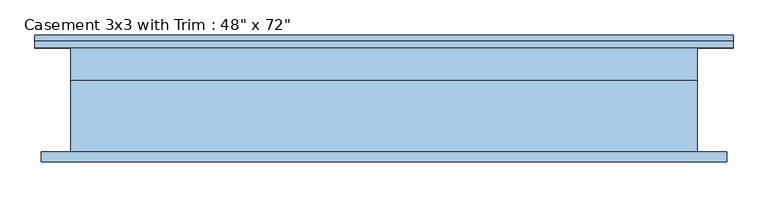
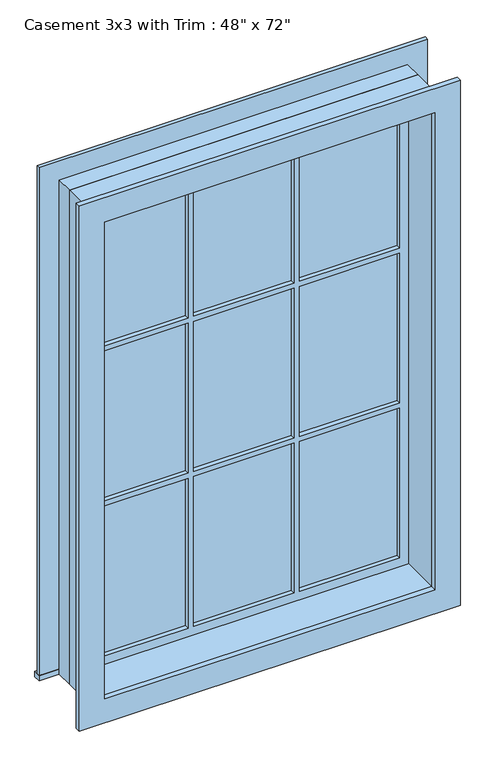
"""IFC4 building model written with IfcOpenShell, lengths in millimetres: window geometry."""

from ifc_helpers import new_model, si_unit, frame, origin, place, context, project, spatial, polyline, outline, extrude, source, transform, mapped, element, save


def window_5a4e61ec(model_context):
    return source(origin(), model_context, "Body", "SweptSolid", [
        extrude(outline(polyline([(-679.45, 127.0), (679.45, 127.0), (679.45, 101.6), (-679.45, 101.6), (-679.45, 127.0)])), frame((0.0, 0.0, 304.8), z_axis=(0.0, 0.0, 1.0), x_axis=(1.0, 0.0, 0.0)), (0.0, 0.0, 1.0), 19.05),
        extrude(outline(polyline([(2114.55, -590.55), (2114.55, 590.55), (323.85, 590.55), (323.85, 679.45), (2203.45, 679.45), (2203.45, -679.45), (323.85, -679.45), (323.85, -590.55), (2114.55, -590.55)])), frame((0.0, 101.6, 0.0), z_axis=(0.0, 1.0, 0.0), x_axis=(0.0, 0.0, 1.0)), (0.0, 0.0, 1.0), 12.7),
        extrude(outline(polyline([(194.7333333, 66.675), (546.1, 66.675), (546.1, 53.975), (194.7333333, 53.975), (194.7333333, 66.675)])), frame((0.0, 0.0, 1515.5333333), z_axis=(0.0, 0.0, 1.0), x_axis=(1.0, 0.0, 0.0)), (0.0, 0.0, 1.0), 554.5666667),
        extrude(outline(polyline([(-175.6833333, 66.675), (175.6833333, 66.675), (175.6833333, 53.975), (-175.6833333, 53.975), (-175.6833333, 66.675)])), frame((0.0, 0.0, 1515.5333333), z_axis=(0.0, 0.0, 1.0), x_axis=(1.0, 0.0, 0.0)), (0.0, 0.0, 1.0), 554.5666667),
        extrude(outline(polyline([(-546.1, 66.675), (-194.7333333, 66.675), (-194.7333333, 53.975), (-546.1, 53.975), (-546.1, 66.675)])), frame((0.0, 0.0, 1515.5333333), z_axis=(0.0, 0.0, 1.0), x_axis=(1.0, 0.0, 0.0)), (0.0, 0.0, 1.0), 554.5666667),
        extrude(outline(polyline([(-546.1, 66.675), (-194.7333333, 66.675), (-194.7333333, 53.975), (-546.1, 53.975), (-546.1, 66.675)])), frame((0.0, 0.0, 941.9166667), z_axis=(0.0, 0.0, 1.0), x_axis=(1.0, 0.0, 0.0)), (0.0, 0.0, 1.0), 554.5666667),
        extrude(outline(polyline([(-175.6833333, 66.675), (175.6833333, 66.675), (175.6833333, 53.975), (-175.6833333, 53.975), (-175.6833333, 66.675)])), frame((0.0, 0.0, 941.9166667), z_axis=(0.0, 0.0, 1.0), x_axis=(1.0, 0.0, 0.0)), (0.0, 0.0, 1.0), 554.5666667),
        extrude(outline(polyline([(194.7333333, 66.675), (546.1, 66.675), (546.1, 53.975), (194.7333333, 53.975), (194.7333333, 66.675)])), frame((0.0, 0.0, 941.9166667), z_axis=(0.0, 0.0, 1.0), x_axis=(1.0, 0.0, 0.0)), (0.0, 0.0, 1.0), 554.5666667),
        extrude(outline(polyline([(194.7333333, 66.675), (546.1, 66.675), (546.1, 53.975), (194.7333333, 53.975), (194.7333333, 66.675)])), frame((0.0, 0.0, 368.3), z_axis=(0.0, 0.0, 1.0), x_axis=(1.0, 0.0, 0.0)), (0.0, 0.0, 1.0), 554.5666667),
        extrude(outline(polyline([(-175.6833333, 66.675), (175.6833333, 66.675), (175.6833333, 53.975), (-175.6833333, 53.975), (-175.6833333, 66.675)])), frame((0.0, 0.0, 368.3), z_axis=(0.0, 0.0, 1.0), x_axis=(1.0, 0.0, 0.0)), (0.0, 0.0, 1.0), 554.5666667),
        extrude(outline(polyline([(-546.1, 66.675), (-194.7333333, 66.675), (-194.7333333, 53.975), (-546.1, 53.975), (-546.1, 66.675)])), frame((0.0, 0.0, 368.3), z_axis=(0.0, 0.0, 1.0), x_axis=(1.0, 0.0, 0.0)), (0.0, 0.0, 1.0), 554.5666667),
        extrude(outline(polyline([(2190.75, 666.75), (2190.75, -666.75), (247.65, -666.75), (247.65, 666.75), (2190.75, 666.75)]), holes=[polyline([(2101.85, 577.85), (336.55, 577.85), (336.55, -577.85), (2101.85, -577.85), (2101.85, 577.85)])]), frame((0.0, -120.65, 0.0), z_axis=(0.0, 1.0, 0.0), x_axis=(0.0, 0.0, 1.0)), (0.0, 0.0, 1.0), 19.05),
        extrude(outline(polyline([(2114.55, -590.55), (323.85, -590.55), (323.85, 590.55), (2114.55, 590.55), (2114.55, -590.55)]), holes=[polyline([(2070.1, -194.7333333), (1515.5333333, -194.7333333), (1515.5333333, -546.1), (2070.1, -546.1), (2070.1, -194.7333333)]), polyline([(1496.4833333, -194.7333333), (941.9166667, -194.7333333), (941.9166667, -546.1), (1496.4833333, -546.1), (1496.4833333, -194.7333333)]), polyline([(922.8666667, -194.7333333), (368.3, -194.7333333), (368.3, -546.1), (922.8666667, -546.1), (922.8666667, -194.7333333)]), polyline([(2070.1, 175.6833333), (1515.5333333, 175.6833333), (1515.5333333, -175.6833333), (2070.1, -175.6833333), (2070.1, 175.6833333)]), polyline([(1496.4833333, 175.6833333), (941.9166667, 175.6833333), (941.9166667, -175.6833333), (1496.4833333, -175.6833333), (1496.4833333, 175.6833333)]), polyline([(922.8666667, 175.6833333), (368.3, 175.6833333), (368.3, -175.6833333), (922.8666667, -175.6833333), (922.8666667, 175.6833333)]), polyline([(2070.1, 546.1), (1515.5333333, 546.1), (1515.5333333, 194.7333333), (2070.1, 194.7333333), (2070.1, 546.1)]), polyline([(1496.4833333, 546.1), (941.9166667, 546.1), (941.9166667, 194.7333333), (1496.4833333, 194.7333333), (1496.4833333, 546.1)]), polyline([(922.8666667, 546.1), (368.3, 546.1), (368.3, 194.7333333), (922.8666667, 194.7333333), (922.8666667, 546.1)])]), frame((0.0, 38.1, 0.0), z_axis=(0.0, 1.0, 0.0), x_axis=(0.0, 0.0, 1.0)), (0.0, 0.0, 1.0), 44.45),
        extrude(outline(polyline([(2133.6, -609.6), (304.8, -609.6), (304.8, 609.6), (2133.6, 609.6), (2133.6, -609.6)]), holes=[polyline([(2101.85, -577.85), (2101.85, 577.85), (336.55, 577.85), (336.55, -577.85), (2101.85, -577.85)])]), frame((0.0, -101.6, 0.0), z_axis=(0.0, 1.0, 0.0), x_axis=(0.0, 0.0, 1.0)), (0.0, 0.0, 1.0), 139.7),
        extrude(outline(polyline([(2133.6, 609.6), (2133.6, -609.6), (304.8, -609.6), (304.8, 609.6), (2133.6, 609.6)]), holes=[polyline([(2114.55, 590.55), (323.85, 590.55), (323.85, -590.55), (2114.55, -590.55), (2114.55, 590.55)])]), frame((0.0, 38.1, 0.0), z_axis=(0.0, 1.0, 0.0), x_axis=(0.0, 0.0, 1.0)), (0.0, 0.0, 1.0), 63.5),
    ])


if __name__ == "__main__":
    model = new_model("IFC4")
    model_context = context("Model", 3, world=origin())
    ifc_project = project(units=[si_unit("LENGTHUNIT", "METRE", prefix="MILLI")], contexts=[model_context])
    site = spatial("IfcSite", under=ifc_project)
    building = spatial("IfcBuilding", under=site)
    placement = place(None, origin())
    window_shape = window_5a4e61ec(model_context)
    element("IfcWindow", 1, ObjectType="Casement 3x3 with Trim : 48\" x 72\"", at=placement, inside=building, context=model_context, shape_type="MappedRepresentation", body=[
        mapped(window_shape, transform((0.0, 0.0, 0.0), x_axis=(1.0, 0.0, 0.0), y_axis=(0.0, 1.0, 0.0), z_axis=(0.0, 0.0, 1.0))),
    ])
    save(model, "model.ifc")

# Revit data of these elements
# Type "Casement 3x3 with Trim : 48\" x 72\""
#   Type Mark = "12"
#   Construction Type Id = "GSP4R"
#   Assembly Code = "B2020100"
#   Analytic Construction = "1/8 in Pilkington single glazing"
#   Visual Light Transmittance = 0.9
#   Solar Heat Gain Coefficient = 0.78
#   Heat Transfer Coefficient (U) = 0.6496 BTU/(h·ft²·°F)
#   Height = 6' - 0"
#   Default Sill Height = 1' - 0"
#   Trim Projection - Ext. = 0' - 0 1/2"
#   Trim Projection - Int. = 0' - 0 3/4"
#   Trim Width - Exterior = 0' - 3 1/2"
#   Trim Width - Interior = 0' - 3 1/2"
#   Width = 4' - 0"
#   Window Inset = 0' - 0 3/4"
#   Define Thermal Properties by = 1
#   Glass Pane Material = Glass
#   Sash Material = Sash
#   Trim Exterior Material = Trim
#   Trim Interior Material = Trim
#   Wall Closure = (empty or 0)
# Element 1 (IfcWindow, "Casement 3x3 with Trim : 48\" x 72\"")
#   Materials on its faces: "Sash", "Glass", "Trim"
# Materials
#   "Glass": class "Glass", colour RGB 0 128 192, transparency 0.75, Description = "Soda Lime Glass", Cost = 0
#   "Sash": class "Wood", colour RGB 224 178 126, transparency 0
#   "Trim": class "Wood", colour RGB 224 178 126, transparency 0
